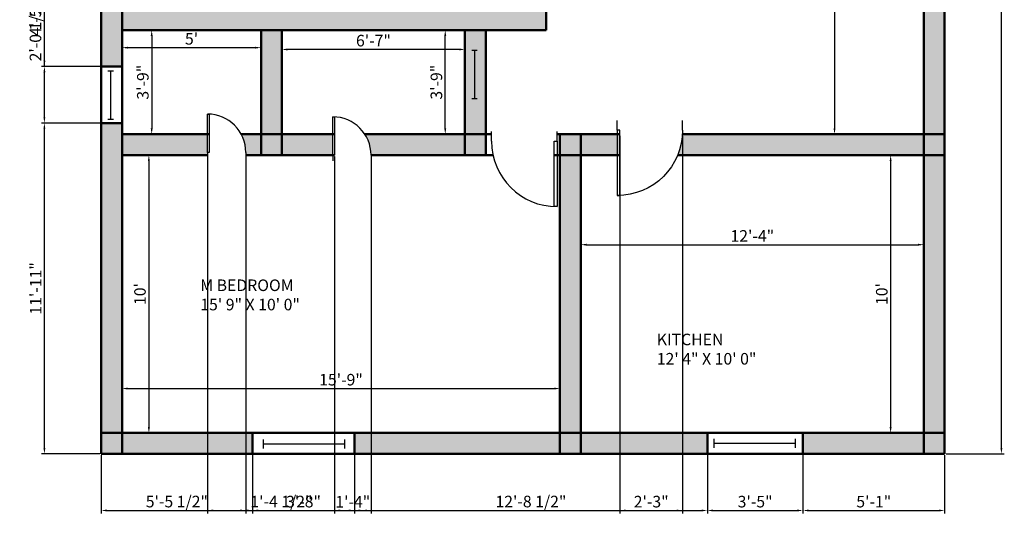
# Model space of a CAD drawing. Units: millimetres. Extents: x 2784 to 3697, y 603 to 1406.
# Tile 8 of 10: x 3272 to 3697, y 737 to 953. Entities that reach past the tile are written whole.
import ezdxf

# ---------------------------------------------------------------- set-up
doc = ezdxf.new("R2010")
doc.units = ezdxf.units.MM
for name, color, linetype, lineweight in [('A-ANNO-DIMS', 140, 'Continuous', 18), ('A-AREA-IDEN', 150, 'Continuous', 25), ('A-DOOR', 10, 'Continuous', 25), ('A-GLAZ', 30, 'Continuous', 25), ('A-WALL', 2, 'Continuous', 50), ('A-WALL-PATT', 8, 'Continuous', 13)]:
    doc.layers.add(name, color=color, linetype=linetype, lineweight=lineweight)
doc.styles.get("Standard").update_dxf_attribs({"font": 'arial.ttf'})
doc.dimstyles.new('ISO-25', dxfattribs={"dimtxt": 5, "dimasz": 2.5, "dimexe": 1.25, "dimexo": 0.625, "dimtad": 1, "dimdec": 0, "dimlunit": 3, "dimtxsty": 'Standard', "dimcen": 2.5, "dimadec": 0, "dimazin": 0, "dimtfac": 1, "dimtdec": 0, "dimtmove": 0, "dimatfit": 3, "dimfxl": 1, "dimarcsym": 0})

# ---------------------------------------------------------------- blocks, each defined once
blk = doc.blocks.new('*U2')
for p, q in [((0, 0), (0, -6)), ((40, 0), (40, -6))]:
    blk.add_line(p, q)
blk.add_lwpolyline([(0, 0), (0, 40), (1.75, 40), (1.75, 0)], close=True)
blk.add_arc((0, 0), 40, 0, 90)
blk = doc.blocks.new('*U38')
for p, q in [((0, 4), (0, 0)), ((0, 2), (36, 2)), ((36, 4), (36, 0))]:
    blk.add_line(p, q)
blk = doc.blocks.new('*D47')
at = {"layer": 'A-ANNO-DIMS', "color": 0, "lineweight": -2, "transparency": 16777216}
for p, q in [((3327.19, 894.31), (3329.06, 894.31)), ((3327.81, 891.81), (3327.81, 776.81)), ((3327.19, 774.31), (3329.06, 774.31))]:
    blk.add_line(p, q, dxfattribs=at)
at = {"layer": 'A-ANNO-DIMS', "color": 0, "transparency": 16777216}
for points in [[(3327.39, 891.81), (3328.23, 891.81), (3327.81, 894.31)], [(3327.39, 776.81), (3328.23, 776.81), (3327.81, 774.31)]]:
    blk.add_solid(points, dxfattribs=at)
at = {"layer": 'Defpoints', "color": 0, "transparency": 16777216}
for p in [(3326.56, 894.31), (3326.56, 774.31), (3327.81, 774.31)]:
    blk.add_point(p, dxfattribs=at)
at = {"layer": 'A-ANNO-DIMS', "color": 0, "transparency": 16777216, "insert": (3324.63, 834.31), "char_height": 5, "attachment_point": 5, "rotation": 90}
blk.add_mtext("10'", dxfattribs=at)
blk = doc.blocks.new('*D48')
at = {"layer": 'A-ANNO-DIMS', "color": 0, "lineweight": -2, "transparency": 16777216}
for p, q in [((3316.23, 794.11), (3316.23, 794.73)), ((3505.23, 794.11), (3505.23, 794.73)), ((3318.73, 793.48), (3502.73, 793.48))]:
    blk.add_line(p, q, dxfattribs=at)
at = {"layer": 'A-ANNO-DIMS', "color": 0, "transparency": 16777216}
for points in [[(3318.73, 793.9), (3318.73, 793.07), (3316.23, 793.48)], [(3502.73, 793.9), (3502.73, 793.07), (3505.23, 793.48)]]:
    blk.add_solid(points, dxfattribs=at)
at = {"layer": 'Defpoints', "color": 0, "transparency": 16777216}
for p in [(3316.23, 793.48), (3505.23, 793.48), (3505.23, 793.48)]:
    blk.add_point(p, dxfattribs=at)
at = {"layer": 'A-ANNO-DIMS', "color": 0, "transparency": 16777216, "insert": (3410.73, 796.66), "char_height": 5, "attachment_point": 5}
blk.add_mtext('15\'-9"', dxfattribs=at)
blk = doc.blocks.new('*D49')
at = {"layer": 'A-ANNO-DIMS', "color": 0, "lineweight": -2, "transparency": 16777216}
for p, q in [((3643.54, 894.31), (3649.17, 894.31)), ((3647.92, 891.81), (3647.92, 776.81)), ((3643.54, 774.31), (3649.17, 774.31))]:
    blk.add_line(p, q, dxfattribs=at)
at = {"layer": 'A-ANNO-DIMS', "color": 0, "transparency": 16777216}
for points in [[(3647.5, 891.81), (3648.33, 891.81), (3647.92, 894.31)], [(3647.5, 776.81), (3648.33, 776.81), (3647.92, 774.31)]]:
    blk.add_solid(points, dxfattribs=at)
at = {"layer": 'Defpoints', "color": 0, "transparency": 16777216}
for p in [(3642.91, 894.31), (3642.91, 774.31), (3647.92, 774.31)]:
    blk.add_point(p, dxfattribs=at)
at = {"layer": 'A-ANNO-DIMS', "color": 0, "transparency": 16777216, "insert": (3644.74, 834.31), "char_height": 5, "attachment_point": 5, "rotation": 90}
blk.add_mtext("10'", dxfattribs=at)
blk = doc.blocks.new('*D50')
at = {"layer": 'A-ANNO-DIMS', "color": 0, "lineweight": -2, "transparency": 16777216}
for p, q in [((3514.23, 859.71), (3514.23, 854.36)), ((3662.23, 859.71), (3662.23, 854.36)), ((3516.73, 855.61), (3659.73, 855.61))]:
    blk.add_line(p, q, dxfattribs=at)
at = {"layer": 'A-ANNO-DIMS', "color": 0, "transparency": 16777216}
for points in [[(3516.73, 856.03), (3516.73, 855.2), (3514.23, 855.61)], [(3659.73, 856.03), (3659.73, 855.2), (3662.23, 855.61)]]:
    blk.add_solid(points, dxfattribs=at)
at = {"layer": 'Defpoints', "color": 0, "transparency": 16777216}
for p in [(3514.23, 860.33), (3662.23, 860.33), (3662.23, 855.61)]:
    blk.add_point(p, dxfattribs=at)
at = {"layer": 'A-ANNO-DIMS', "color": 0, "transparency": 16777216, "insert": (3588.23, 858.75), "char_height": 5, "attachment_point": 5}
blk.add_mtext('12\'-4"', dxfattribs=at)
blk = doc.blocks.new('*D51')
at = {"layer": 'A-ANNO-DIMS', "color": 0, "lineweight": -2, "transparency": 16777216}
for p, q in [((3329.65, 948.31), (3330.28, 948.31)), ((3329.03, 945.81), (3329.03, 905.81)), ((3329.65, 903.31), (3330.28, 903.31))]:
    blk.add_line(p, q, dxfattribs=at)
at = {"layer": 'A-ANNO-DIMS', "color": 0, "transparency": 16777216}
for points in [[(3328.61, 945.81), (3329.44, 945.81), (3329.03, 948.31)], [(3328.61, 905.81), (3329.44, 905.81), (3329.03, 903.31)]]:
    blk.add_solid(points, dxfattribs=at)
at = {"layer": 'Defpoints', "color": 0, "transparency": 16777216}
for p in [(3329.03, 948.31), (3329.03, 903.31), (3329.03, 903.31)]:
    blk.add_point(p, dxfattribs=at)
at = {"layer": 'A-ANNO-DIMS', "color": 0, "transparency": 16777216, "insert": (3325.85, 925.81), "char_height": 5, "attachment_point": 5, "rotation": 90}
blk.add_mtext('3\'-9"', dxfattribs=at)
blk = doc.blocks.new('*D52')
at = {"layer": 'A-ANNO-DIMS', "color": 0, "lineweight": -2, "transparency": 16777216}
for p, q in [((3316.23, 939.95), (3316.23, 941.97)), ((3318.73, 940.72), (3373.73, 940.72)), ((3376.23, 939.95), (3376.23, 941.97))]:
    blk.add_line(p, q, dxfattribs=at)
at = {"layer": 'A-ANNO-DIMS', "color": 0, "transparency": 16777216}
for points in [[(3318.73, 941.13), (3318.73, 940.3), (3316.23, 940.72)], [(3373.73, 941.13), (3373.73, 940.3), (3376.23, 940.72)]]:
    blk.add_solid(points, dxfattribs=at)
at = {"layer": 'Defpoints', "color": 0, "transparency": 16777216}
for p in [(3316.23, 939.32), (3376.23, 940.72), (3376.23, 939.32)]:
    blk.add_point(p, dxfattribs=at)
at = {"layer": 'A-ANNO-DIMS', "color": 0, "transparency": 16777216, "insert": (3346.23, 943.89), "char_height": 5, "attachment_point": 5}
blk.add_mtext("5'", dxfattribs=at)
blk = doc.blocks.new('*D53')
at = {"layer": 'A-ANNO-DIMS', "color": 0, "lineweight": -2, "transparency": 16777216}
for p, q in [((3385.23, 941.18), (3385.23, 938.69)), ((3461.73, 939.94), (3387.73, 939.94)), ((3464.23, 941.18), (3464.23, 938.69))]:
    blk.add_line(p, q, dxfattribs=at)
at = {"layer": 'A-ANNO-DIMS', "color": 0, "transparency": 16777216}
for points in [[(3387.73, 940.36), (3387.73, 939.53), (3385.23, 939.94)], [(3461.73, 940.36), (3461.73, 939.53), (3464.23, 939.94)]]:
    blk.add_solid(points, dxfattribs=at)
at = {"layer": 'Defpoints', "color": 0, "transparency": 16777216}
for p in [(3385.23, 941.8), (3385.23, 939.94), (3464.23, 941.8)]:
    blk.add_point(p, dxfattribs=at)
at = {"layer": 'A-ANNO-DIMS', "color": 0, "transparency": 16777216, "insert": (3424.73, 943.12), "char_height": 5, "attachment_point": 5}
blk.add_mtext('6\'-7"', dxfattribs=at)
blk = doc.blocks.new('*D54')
at = {"layer": 'A-ANNO-DIMS', "color": 0, "lineweight": -2, "transparency": 16777216}
for p, q in [((3455.63, 948.31), (3454.46, 948.31)), ((3455.71, 905.81), (3455.71, 945.81)), ((3455.63, 903.31), (3454.46, 903.31))]:
    blk.add_line(p, q, dxfattribs=at)
at = {"layer": 'A-ANNO-DIMS', "color": 0, "transparency": 16777216}
for points in [[(3455.3, 945.81), (3456.13, 945.81), (3455.71, 948.31)], [(3455.3, 905.81), (3456.13, 905.81), (3455.71, 903.31)]]:
    blk.add_solid(points, dxfattribs=at)
at = {"layer": 'Defpoints', "color": 0, "transparency": 16777216}
for p in [(3455.71, 948.31), (3456.26, 948.31), (3456.26, 903.31)]:
    blk.add_point(p, dxfattribs=at)
at = {"layer": 'A-ANNO-DIMS', "color": 0, "transparency": 16777216, "insert": (3452.54, 925.81), "char_height": 5, "attachment_point": 5, "rotation": 90}
blk.add_mtext('3\'-9"', dxfattribs=at)
blk = doc.blocks.new('*D58')
at = {"layer": 'A-ANNO-DIMS', "color": 0, "lineweight": -2, "transparency": 16777216}
for p, q in [((3624.82, 1095.28), (3622.46, 1095.28)), ((3623.71, 1092.78), (3623.71, 905.81)), ((3624.82, 903.31), (3622.46, 903.31))]:
    blk.add_line(p, q, dxfattribs=at)
at = {"layer": 'A-ANNO-DIMS', "color": 0, "transparency": 16777216}
for points in [[(3623.29, 1092.78), (3624.12, 1092.78), (3623.71, 1095.28)], [(3623.29, 905.81), (3624.12, 905.81), (3623.71, 903.31)]]:
    blk.add_solid(points, dxfattribs=at)
at = {"layer": 'Defpoints', "color": 0, "transparency": 16777216}
for p in [(3625.44, 1095.28), (3623.71, 903.31), (3625.44, 903.31)]:
    blk.add_point(p, dxfattribs=at)
at = {"layer": 'A-ANNO-DIMS', "color": 0, "transparency": 16777216, "insert": (3620.53, 999.3), "char_height": 5, "attachment_point": 5, "rotation": 90}
blk.add_mtext("16'", dxfattribs=at)
blk = doc.blocks.new('*D118')
at = {"layer": 'A-ANNO-DIMS', "color": 0, "lineweight": -2, "transparency": 16777216}
for p, q in [((3307.23, 764.69), (3307.23, 739.56)), ((3372.55, 764.69), (3372.55, 739.56)), ((3309.73, 740.81), (3370.05, 740.81))]:
    blk.add_line(p, q, dxfattribs=at)
at = {"layer": 'A-ANNO-DIMS', "color": 0, "transparency": 16777216}
for points in [[(3309.73, 741.23), (3309.73, 740.39), (3307.23, 740.81)], [(3370.05, 741.23), (3370.05, 740.39), (3372.55, 740.81)]]:
    blk.add_solid(points, dxfattribs=at)
at = {"layer": 'Defpoints', "color": 0, "transparency": 16777216}
for p in [(3307.23, 765.31), (3372.55, 765.31), (3372.55, 740.81)]:
    blk.add_point(p, dxfattribs=at)
at = {"layer": 'A-ANNO-DIMS', "color": 0, "transparency": 16777216, "insert": (3339.89, 744.02), "char_height": 5, "attachment_point": 5}
blk.add_mtext('5\'-5 1/2"', dxfattribs=at)
blk = doc.blocks.new('*D119')
at = {"layer": 'A-ANNO-DIMS', "color": 0, "lineweight": -2, "transparency": 16777216}
for p, q in [((3372.55, 764.69), (3372.55, 739.56)), ((3416.56, 764.69), (3416.56, 739.56)), ((3375.05, 740.81), (3414.06, 740.81))]:
    blk.add_line(p, q, dxfattribs=at)
at = {"layer": 'A-ANNO-DIMS', "color": 0, "transparency": 16777216}
for points in [[(3375.05, 741.23), (3375.05, 740.39), (3372.55, 740.81)], [(3414.06, 741.23), (3414.06, 740.39), (3416.56, 740.81)]]:
    blk.add_solid(points, dxfattribs=at)
at = {"layer": 'Defpoints', "color": 0, "transparency": 16777216}
for p in [(3372.55, 765.31), (3416.56, 765.31), (3416.56, 740.81)]:
    blk.add_point(p, dxfattribs=at)
at = {"layer": 'A-ANNO-DIMS', "color": 0, "transparency": 16777216, "insert": (3394.55, 743.99), "char_height": 5, "attachment_point": 5}
blk.add_mtext('3\'-8"', dxfattribs=at)
blk = doc.blocks.new('*D120')
at = {"layer": 'A-ANNO-DIMS', "color": 0, "lineweight": -2, "transparency": 16777216}
for p, q in [((3416.56, 764.69), (3416.56, 739.56)), ((3568.83, 764.69), (3568.83, 739.56)), ((3419.06, 740.81), (3566.33, 740.81))]:
    blk.add_line(p, q, dxfattribs=at)
at = {"layer": 'A-ANNO-DIMS', "color": 0, "transparency": 16777216}
for points in [[(3419.06, 741.23), (3419.06, 740.39), (3416.56, 740.81)], [(3566.33, 741.23), (3566.33, 740.39), (3568.83, 740.81)]]:
    blk.add_solid(points, dxfattribs=at)
at = {"layer": 'Defpoints', "color": 0, "transparency": 16777216}
for p in [(3416.56, 765.31), (3568.83, 765.31), (3568.83, 740.81)]:
    blk.add_point(p, dxfattribs=at)
at = {"layer": 'A-ANNO-DIMS', "color": 0, "transparency": 16777216, "insert": (3492.69, 744.02), "char_height": 5, "attachment_point": 5}
blk.add_mtext('12\'-8 1/2"', dxfattribs=at)
blk = doc.blocks.new('*D121')
at = {"layer": 'A-ANNO-DIMS', "color": 0, "lineweight": -2, "transparency": 16777216}
for p, q in [((3568.83, 764.69), (3568.83, 739.56)), ((3610.06, 764.69), (3610.06, 739.56)), ((3571.33, 740.81), (3607.56, 740.81))]:
    blk.add_line(p, q, dxfattribs=at)
at = {"layer": 'A-ANNO-DIMS', "color": 0, "transparency": 16777216}
for points in [[(3571.33, 741.23), (3571.33, 740.39), (3568.83, 740.81)], [(3607.56, 741.23), (3607.56, 740.39), (3610.06, 740.81)]]:
    blk.add_solid(points, dxfattribs=at)
at = {"layer": 'Defpoints', "color": 0, "transparency": 16777216}
for p in [(3568.83, 765.31), (3610.06, 765.31), (3610.06, 740.81)]:
    blk.add_point(p, dxfattribs=at)
at = {"layer": 'A-ANNO-DIMS', "color": 0, "transparency": 16777216, "insert": (3589.44, 743.99), "char_height": 5, "attachment_point": 5}
blk.add_mtext('3\'-5"', dxfattribs=at)
blk = doc.blocks.new('*D122')
at = {"layer": 'A-ANNO-DIMS', "color": 0, "lineweight": -2, "transparency": 16777216}
for p, q in [((3610.06, 764.69), (3610.06, 739.56)), ((3671.23, 764.69), (3671.23, 739.56)), ((3612.56, 740.81), (3668.73, 740.81))]:
    blk.add_line(p, q, dxfattribs=at)
at = {"layer": 'A-ANNO-DIMS', "color": 0, "transparency": 16777216}
for points in [[(3612.56, 741.23), (3612.56, 740.39), (3610.06, 740.81)], [(3668.73, 741.23), (3668.73, 740.39), (3671.23, 740.81)]]:
    blk.add_solid(points, dxfattribs=at)
at = {"layer": 'Defpoints', "color": 0, "transparency": 16777216}
for p in [(3610.06, 765.31), (3671.23, 765.31), (3671.23, 740.81)]:
    blk.add_point(p, dxfattribs=at)
at = {"layer": 'A-ANNO-DIMS', "color": 0, "transparency": 16777216, "insert": (3640.64, 743.99), "char_height": 5, "attachment_point": 5}
blk.add_mtext('5\'-1"', dxfattribs=at)
blk = doc.blocks.new('*D123')
at = {"layer": 'A-ANNO-DIMS', "color": 0, "lineweight": -2, "transparency": 16777216}
for p, q in [((3306.6, 908.17), (3281.48, 908.17)), ((3282.73, 767.81), (3282.73, 905.67)), ((3306.6, 765.31), (3281.48, 765.31))]:
    blk.add_line(p, q, dxfattribs=at)
at = {"layer": 'A-ANNO-DIMS', "color": 0, "transparency": 16777216}
for points in [[(3282.31, 905.67), (3283.14, 905.67), (3282.73, 908.17)], [(3282.31, 767.81), (3283.14, 767.81), (3282.73, 765.31)]]:
    blk.add_solid(points, dxfattribs=at)
at = {"layer": 'Defpoints', "color": 0, "transparency": 16777216}
for p in [(3282.73, 908.17), (3307.23, 908.17), (3307.23, 765.31)]:
    blk.add_point(p, dxfattribs=at)
at = {"layer": 'A-ANNO-DIMS', "color": 0, "transparency": 16777216, "insert": (3279.59, 836.74), "char_height": 5, "attachment_point": 5, "rotation": 90}
blk.add_mtext('11\'-11"', dxfattribs=at)
blk = doc.blocks.new('*D124')
at = {"layer": 'A-ANNO-DIMS', "color": 0, "lineweight": -2, "transparency": 16777216}
for p, q in [((3282.73, 932.57), (3282.73, 961.35)), ((3306.6, 932.57), (3281.48, 932.57)), ((3282.73, 910.67), (3282.73, 930.07)), ((3306.6, 908.17), (3281.48, 908.17))]:
    blk.add_line(p, q, dxfattribs=at)
at = {"layer": 'A-ANNO-DIMS', "color": 0, "transparency": 16777216}
for points in [[(3282.31, 930.07), (3283.14, 930.07), (3282.73, 932.57)], [(3282.31, 910.67), (3283.14, 910.67), (3282.73, 908.17)]]:
    blk.add_solid(points, dxfattribs=at)
at = {"layer": 'Defpoints', "color": 0, "transparency": 16777216}
for p in [(3282.73, 932.57), (3307.23, 932.57), (3307.23, 908.17)]:
    blk.add_point(p, dxfattribs=at)
at = {"layer": 'A-ANNO-DIMS', "color": 0, "transparency": 16777216, "insert": (3279.52, 948.21), "char_height": 5, "attachment_point": 5, "rotation": 90}
blk.add_mtext('2\'-0 1/2"', dxfattribs=at)
blk = doc.blocks.new('*D125')
at = {"layer": 'A-ANNO-DIMS', "color": 0, "lineweight": -2, "transparency": 16777216}
for p, q in [((3306.6, 985.84), (3281.48, 985.84)), ((3282.73, 935.07), (3282.73, 983.34)), ((3306.6, 932.57), (3281.48, 932.57))]:
    blk.add_line(p, q, dxfattribs=at)
at = {"layer": 'A-ANNO-DIMS', "color": 0, "transparency": 16777216}
for points in [[(3282.31, 983.34), (3283.14, 983.34), (3282.73, 985.84)], [(3282.31, 935.07), (3283.14, 935.07), (3282.73, 932.57)]]:
    blk.add_solid(points, dxfattribs=at)
at = {"layer": 'Defpoints', "color": 0, "transparency": 16777216}
for p in [(3282.73, 985.84), (3307.23, 985.84), (3307.23, 932.57)]:
    blk.add_point(p, dxfattribs=at)
at = {"layer": 'A-ANNO-DIMS', "color": 0, "transparency": 16777216, "insert": (3279.52, 959.21), "char_height": 5, "attachment_point": 5, "rotation": 90}
blk.add_mtext('4\'-5 1/2"', dxfattribs=at)
blk = doc.blocks.new('*D130')
at = {"layer": 'A-ANNO-DIMS', "color": 0, "lineweight": -2, "transparency": 16777216}
for p, q in [((3671.85, 1233.28), (3696.98, 1233.28)), ((3695.73, 767.81), (3695.73, 1230.78)), ((3671.85, 765.31), (3696.98, 765.31))]:
    blk.add_line(p, q, dxfattribs=at)
at = {"layer": 'A-ANNO-DIMS', "color": 0, "transparency": 16777216}
for points in [[(3695.31, 1230.78), (3696.14, 1230.78), (3695.73, 1233.28)], [(3695.31, 767.81), (3696.14, 767.81), (3695.73, 765.31)]]:
    blk.add_solid(points, dxfattribs=at)
at = {"layer": 'Defpoints', "color": 0, "transparency": 16777216}
for p in [(3671.23, 1233.28), (3695.73, 1233.28), (3671.23, 765.31)]:
    blk.add_point(p, dxfattribs=at)
at = {"layer": 'A-ANNO-DIMS', "color": 0, "transparency": 16777216, "insert": (3692.55, 999.3), "char_height": 5, "attachment_point": 5, "rotation": 90}
blk.add_mtext('39\'-0"', dxfattribs=at)
blk = doc.blocks.new('*D136')
at = {"layer": 'A-ANNO-DIMS', "color": 0, "lineweight": -2, "transparency": 16777216}
for p, q in [((3353.12, 893.69), (3353.12, 739.56)), ((3369.65, 893.69), (3369.65, 739.56)), ((3355.62, 740.81), (3367.15, 740.81)), ((3369.65, 740.81), (3397.87, 740.81))]:
    blk.add_line(p, q, dxfattribs=at)
at = {"layer": 'A-ANNO-DIMS', "color": 0, "transparency": 16777216}
for points in [[(3355.62, 741.23), (3355.62, 740.39), (3353.12, 740.81)], [(3367.15, 741.23), (3367.15, 740.39), (3369.65, 740.81)]]:
    blk.add_solid(points, dxfattribs=at)
at = {"layer": 'Defpoints', "color": 0, "transparency": 16777216}
for p in [(3353.12, 894.31), (3369.65, 894.31), (3369.65, 740.81)]:
    blk.add_point(p, dxfattribs=at)
at = {"layer": 'A-ANNO-DIMS', "color": 0, "transparency": 16777216, "insert": (3385.01, 744.02), "char_height": 5, "attachment_point": 5}
blk.add_mtext('1\'-4 1/2"', dxfattribs=at)
blk = doc.blocks.new('*D137')
at = {"layer": 'A-ANNO-DIMS', "color": 0, "lineweight": -2, "transparency": 16777216}
for p, q in [((3407.89, 893.69), (3407.89, 739.56)), ((3423.7, 893.69), (3423.7, 739.56)), ((3410.39, 740.81), (3421.2, 740.81))]:
    blk.add_line(p, q, dxfattribs=at)
at = {"layer": 'A-ANNO-DIMS', "color": 0, "transparency": 16777216}
for points in [[(3410.39, 741.23), (3410.39, 740.39), (3407.89, 740.81)], [(3421.2, 741.23), (3421.2, 740.39), (3423.7, 740.81)]]:
    blk.add_solid(points, dxfattribs=at)
at = {"layer": 'Defpoints', "color": 0, "transparency": 16777216}
for p in [(3407.89, 894.31), (3423.7, 894.31), (3423.7, 740.81)]:
    blk.add_point(p, dxfattribs=at)
at = {"layer": 'A-ANNO-DIMS', "color": 0, "transparency": 16777216, "insert": (3415.8, 743.95), "char_height": 5, "attachment_point": 5}
blk.add_mtext('1\'-4"', dxfattribs=at)
blk = doc.blocks.new('*D138')
at = {"layer": 'A-ANNO-DIMS', "color": 0, "lineweight": -2, "transparency": 16777216}
for p, q in [((3531.12, 902.69), (3531.12, 739.56)), ((3558.05, 902.69), (3558.05, 739.56)), ((3533.62, 740.81), (3555.55, 740.81))]:
    blk.add_line(p, q, dxfattribs=at)
at = {"layer": 'A-ANNO-DIMS', "color": 0, "transparency": 16777216}
for points in [[(3533.62, 741.23), (3533.62, 740.39), (3531.12, 740.81)], [(3555.55, 741.23), (3555.55, 740.39), (3558.05, 740.81)]]:
    blk.add_solid(points, dxfattribs=at)
at = {"layer": 'Defpoints', "color": 0, "transparency": 16777216}
for p in [(3531.12, 903.31), (3558.05, 903.31), (3558.05, 740.81)]:
    blk.add_point(p, dxfattribs=at)
at = {"layer": 'A-ANNO-DIMS', "color": 0, "transparency": 16777216, "insert": (3544.59, 743.99), "char_height": 5, "attachment_point": 5}
blk.add_mtext('2\'-3"', dxfattribs=at)

msp = doc.modelspace()

# ---------------------------------------------------------------- hatches: boundary and pattern name
at = {"layer": 'A-WALL-PATT'}
h = msp.add_hatch(color=256, dxfattribs=at)
h.dxf.hatch_style = 1
h.paths.add_polyline_path([(3316.23, 1224.28), (3307.23, 1224.28), (3307.23, 1104.28), (3316.23, 1104.28)])
h.paths.add_polyline_path([(3316.23, 1233.28), (3307.23, 1233.28), (3307.23, 1224.28), (3316.23, 1224.28)])
h.paths.add_polyline_path([(3363.37, 1233.28), (3316.23, 1233.28), (3316.23, 1224.28), (3363.37, 1224.28)])
h.paths.add_polyline_path([(3460.23, 1233.28), (3405.1, 1233.28), (3405.1, 1224.28), (3460.23, 1224.28)])
h.paths.add_polyline_path([(3469.23, 1233.28), (3460.23, 1233.28), (3460.23, 1224.28), (3469.23, 1224.28)])
h.paths.add_polyline_path([(3469.23, 1224.28), (3460.23, 1224.28), (3460.23, 1104.28), (3469.23, 1104.28)])
h.paths.add_polyline_path([(3469.23, 1104.28), (3460.23, 1104.28), (3460.23, 1095.28), (3469.23, 1095.28)])
h.paths.add_polyline_path([(3460.23, 1104.28), (3444.39, 1104.28), (3444.39, 1097.52), (3444.39, 1095.28), (3460.23, 1095.28)])
h.paths.add_polyline_path([(3409.23, 1095.28), (3400.23, 1095.28), (3400.23, 1066.17, -0.119943), (3407.82, 1068.02), (3409.23, 1068.02)])
h.paths.add_polyline_path([(3409.23, 1104.28), (3400.23, 1104.28), (3400.23, 1095.28), (3409.23, 1095.28)])
h.paths.add_polyline_path([(3400.23, 1104.28), (3316.23, 1104.28), (3316.23, 1095.28), (3400.23, 1095.28)])
h.paths.add_polyline_path([(3316.23, 1104.28), (3307.23, 1104.28), (3307.23, 1095.28), (3316.23, 1095.28)])
h.paths.add_polyline_path([(3316.23, 1095.28), (3307.23, 1095.28), (3307.23, 1083.49), (3316.23, 1083.49)])
h.paths.add_polyline_path([(3416.17, 1097.52, -0.060509), (3416.99, 1104.28), (3409.23, 1104.28), (3409.23, 1095.28), (3416.17, 1095.28)])
h.paths.add_polyline_path([(3538.23, 1224.28), (3529.23, 1224.28), (3529.23, 1104.28), (3538.23, 1104.28)])
h.paths.add_polyline_path([(3538.23, 1233.28), (3529.23, 1233.28), (3529.23, 1224.28), (3538.23, 1224.28)])
h.paths.add_polyline_path([(3529.23, 1233.28), (3510.77, 1233.28), (3510.77, 1224.28), (3529.23, 1224.28)])
h.paths.add_polyline_path([(3483.89, 1233.28), (3469.23, 1233.28), (3469.23, 1224.28), (3483.89, 1224.28)])
h.paths.add_polyline_path([(3662.23, 1233.28), (3629.82, 1233.28), (3629.82, 1224.28), (3662.23, 1224.28)])
h.paths.add_polyline_path([(3671.23, 1233.28), (3662.23, 1233.28), (3662.23, 1224.28), (3671.23, 1224.28)])
h.paths.add_polyline_path([(3671.23, 1224.28), (3662.23, 1224.28), (3662.23, 1104.28), (3671.23, 1104.28)])
h.paths.add_polyline_path([(3588.37, 1233.28), (3538.23, 1233.28), (3538.23, 1224.28), (3588.37, 1224.28)])
h.paths.add_polyline_path([(3662.23, 1104.28), (3579.01, 1104.28, -0.053945), (3579.66, 1098.24), (3579.66, 1095.28), (3662.23, 1095.28)])
h.paths.add_polyline_path([(3671.23, 1104.28), (3662.23, 1104.28), (3662.23, 1095.28), (3671.23, 1095.28)])
h.paths.add_polyline_path([(3551.44, 1104.28), (3538.23, 1104.28), (3538.23, 1095.28), (3551.44, 1095.28), (3551.44, 1098.24)])
h.paths.add_polyline_path([(3538.23, 1104.28), (3529.23, 1104.28), (3529.23, 1095.28), (3538.23, 1095.28)])
h.paths.add_polyline_path([(3671.23, 1095.28), (3662.23, 1095.28), (3662.23, 903.31), (3671.23, 903.31)])
h.paths.add_polyline_path([(3316.23, 985.84), (3307.23, 985.84), (3307.23, 932.57), (3316.23, 932.57)])
h.paths.add_polyline_path([(3316.23, 1041.28), (3307.23, 1041.28), (3307.23, 1012.14), (3316.23, 1012.14)])
h.paths.add_polyline_path([(3316.23, 1050.28), (3307.23, 1050.28), (3307.23, 1041.28), (3316.23, 1041.28)])
h.paths.add_polyline_path([(3400.23, 1050.28), (3316.23, 1050.28), (3316.23, 1041.28), (3400.23, 1041.28)])
h.paths.add_polyline_path([(3316.23, 1059.19), (3307.23, 1059.19), (3307.23, 1050.28), (3316.23, 1050.28)])
h.paths.add_polyline_path([(3316.23, 908.17), (3307.23, 908.17), (3307.23, 774.31), (3316.23, 774.31)])
h.paths.add_polyline_path([(3316.23, 774.31), (3307.23, 774.31), (3307.23, 765.31), (3316.23, 765.31)])
h.paths.add_polyline_path([(3372.55, 774.31), (3316.23, 774.31), (3316.23, 765.31), (3372.55, 765.31)])
h.paths.add_polyline_path([(3505.23, 774.31), (3416.56, 774.31), (3416.56, 765.31), (3505.23, 765.31)])
h.paths.add_polyline_path([(3568.83, 774.31), (3514.23, 774.31), (3514.23, 765.31), (3568.83, 765.31)])
h.paths.add_polyline_path([(3514.23, 774.31), (3505.23, 774.31), (3505.23, 765.31), (3514.23, 765.31)])
h.paths.add_polyline_path([(3514.23, 894.31), (3505.23, 894.31), (3505.23, 774.31), (3514.23, 774.31)])
h.paths.add_polyline_path([(3514.23, 903.31), (3505.23, 903.31), (3505.23, 894.31), (3514.23, 894.31)])
h.paths.add_polyline_path([(3473.23, 948.31), (3464.23, 948.31), (3464.23, 903.31), (3473.23, 903.31)])
h.paths.add_polyline_path([(3473.23, 903.31), (3464.23, 903.31), (3464.23, 894.31), (3473.23, 894.31)])
h.paths.add_polyline_path([(3464.23, 903.31), (3421.03, 903.31, -0.144956), (3423.7, 894.31), (3464.23, 894.31)])
h.paths.add_polyline_path([(3385.23, 903.31), (3376.23, 903.31), (3376.23, 894.31), (3385.23, 894.31)])
h.paths.add_polyline_path([(3385.23, 948.31), (3376.23, 948.31), (3376.23, 903.31), (3385.23, 903.31)])
h.paths.add_polyline_path([(3407.17, 903.31), (3385.23, 903.31), (3385.23, 894.31), (3407.17, 894.31)])
h.paths.add_polyline_path([(3353.12, 903.31), (3316.23, 903.31), (3316.23, 894.31), (3353.12, 894.31), (3353.12, 895.49)])
h.paths.add_polyline_path([(3376.23, 903.31), (3367.68, 903.31, -0.123903), (3369.65, 895.49), (3369.65, 894.31), (3376.23, 894.31)])
h.paths.add_polyline_path([(3499.23, 957.31), (3499.23, 1041.28), (3490.23, 1041.28), (3490.23, 957.31), (3316.23, 957.31), (3316.23, 948.31), (3490.23, 948.31), (3499.23, 948.31)])
h.paths.add_polyline_path([(3490.23, 1050.28), (3485.56, 1050.28), (3409.23, 1050.28), (3409.23, 1041.28), (3490.23, 1041.28)])
h.paths.add_polyline_path([(3409.23, 1050.28), (3400.23, 1050.28), (3400.23, 1041.28), (3409.23, 1041.28)])
h.paths.add_polyline_path([(3499.23, 1050.28), (3490.23, 1050.28), (3490.23, 1041.28), (3499.23, 1041.28)])
h.paths.add_polyline_path([(3671.23, 894.31), (3662.23, 894.31), (3662.23, 774.31), (3671.23, 774.31)])
h.paths.add_polyline_path([(3671.23, 903.31), (3662.23, 903.31), (3662.23, 894.31), (3671.23, 894.31)])
h.paths.add_polyline_path([(3662.23, 903.31), (3558.05, 903.31, -0.082354), (3555.98, 894.31), (3662.23, 894.31)])
h.paths.add_polyline_path([(3529.88, 903.31), (3514.23, 903.31), (3514.23, 894.31), (3529.88, 894.31)])
h.paths.add_polyline_path([(3531.12, 903.31), (3529.88, 903.31), (3529.88, 894.31), (3531.12, 894.31)])
h.paths.add_polyline_path([(3662.23, 774.31), (3610.06, 774.31), (3610.06, 765.31), (3662.23, 765.31)])
h.paths.add_polyline_path([(3671.23, 774.31), (3662.23, 774.31), (3662.23, 765.31), (3671.23, 765.31)])
h.paths.add_polyline_path([(3544.99, 801.01), (3590.84, 801.01), (3590.84, 819.67), (3544.99, 819.67)], flags=9)
h.paths.add_polyline_path([(3347.99, 824.43), (3394.58, 824.43), (3394.58, 843.09), (3347.99, 843.09)], flags=9)
h.paths.add_polyline_path([(3546.35, 988.53), (3592.21, 988.53), (3592.21, 1007.19), (3546.35, 1007.19)], flags=9)
h.paths.add_polyline_path([(3329.63, 1060.44), (3367.72, 1060.44), (3367.72, 1079.1), (3329.63, 1079.1)], flags=9)
h.paths.add_polyline_path([(3353.92, 1169.75), (3400.92, 1169.75), (3400.92, 1188.4), (3353.92, 1188.4)], flags=9)

# ---------------------------------------------------------------- linework, layer by layer
at = {"layer": 'A-WALL'}
for p, q in [((3307.23, 1233.28), (3307.23, 765.31)), ((3316.23, 1233.28), (3316.23, 765.31)), ((3662.23, 1233.28), (3662.23, 765.31)), ((3671.23, 1233.28), (3671.23, 765.31)), ((3499.23, 948.31), (3499.23, 957.31)), ((3316.23, 948.31), (3490.23, 948.31)), ((3376.23, 948.31), (3376.23, 894.31)), ((3385.23, 948.31), (3385.23, 894.31)), ((3464.23, 948.31), (3464.23, 894.31)), ((3473.23, 948.31), (3473.23, 894.31)), ((3490.23, 948.31), (3499.23, 948.31)), ((3316.23, 932.57), (3307.23, 932.57)), ((3316.23, 908.17), (3307.23, 908.17)), ((3316.23, 903.31), (3353.84, 903.31)), ((3367.68, 903.31), (3407.89, 903.31)), ((3421.03, 903.31), (3475.73, 903.31)), ((3503.95, 903.31), (3531.12, 903.31)), ((3505.23, 903.31), (3505.23, 765.31)), ((3514.23, 903.31), (3514.23, 765.31)), ((3558.05, 903.31), (3671.23, 903.31)), ((3316.23, 894.31), (3353.12, 894.31)), ((3369.65, 894.31), (3407.89, 894.31)), ((3423.7, 894.31), (3476.36, 894.31)), ((3502.72, 894.31), (3531.12, 894.31)), ((3555.98, 894.31), (3671.23, 894.31)), ((3307.23, 774.31), (3671.23, 774.31)), ((3372.55, 774.31), (3372.55, 765.31)), ((3416.56, 774.31), (3416.56, 765.31)), ((3568.83, 774.31), (3568.83, 765.31)), ((3610.06, 774.31), (3610.06, 765.31)), ((3307.23, 765.31), (3671.23, 765.31))]:
    msp.add_line(p, q, dxfattribs=at)

# ---------------------------------------------------------------- block references
at = {"layer": 'A-DOOR', "xscale": 0.413209421180039, "yscale": 0.413209421180039, "zscale": 0.413209421180039}
for p in [(3353.12, 895.49), (3407.17, 894.31)]:
    msp.add_blockref('*U2', p, dxfattribs=at)
at = {"layer": 'A-DOOR', "yscale": 0.7055841571326333, "zscale": 0.7055841571326333, "rotation": 180}
for p, xscale in [((3529.88, 905.05), -0.7055841571326333), ((3503.95, 900.27), 0.7055841571326333)]:
    msp.add_blockref('*U2', p, dxfattribs=dict(at, xscale=xscale))
at = {"layer": 'A-GLAZ', "xscale": 0.5811470115210491, "yscale": 0.5811470115210491, "zscale": 0.5811470115210491, "rotation": 269.9999999999999}
for p in [(3467.2, 939.55), (3310.15, 930.58)]:
    msp.add_blockref('*U38', p, dxfattribs=at)
at = {"layer": 'A-GLAZ', "xscale": 0.9748873049904094, "yscale": 0.9748873049904094, "zscale": 0.9748873049904094}
for p in [(3377.12, 767.64), (3571.6, 767.93)]:
    msp.add_blockref('*U38', p, dxfattribs=at)

# ---------------------------------------------------------------- texts
at = {"layer": 'A-AREA-IDEN', "char_height": 5, "attachment_point": 1}
for s, width, insert in [('M BEDROOM \\P15\' 9" X 10\' 0"', 131.4901, (3350, 840.6)), ('KITCHEN \\P12\' 4" X 10\' 0"', 63.7234, (3547, 817.18))]:
    msp.add_mtext_dynamic_manual_height_columns(s, width=width, gutter_width=12.5, heights=[0], dxfattribs=dict(at, insert=insert))

# ---------------------------------------------------------------- dimensions: what is measured, and where the dimension line sits
at = {"layer": 'A-ANNO-DIMS'}
for base, p1, p2, override, picture, middle in [((3695.73, 1233.28), (3671.23, 765.31), (3671.23, 1233.28), {"dimdec": 1, "dimlfac": 1, "dimrnd": 0, "dimzin": 1, "dimdsep": 46, "dimlunit": 4, "dimfrac": 2}, '*D130', (3692.55, 999.3)), ((3623.71, 903.31), (3625.44, 1095.28), (3625.44, 903.31), {"dimclrd": 0, "dimclre": 0, "dimclrt": 0}, '*D58', (3620.53, 999.3)), ((3282.73, 985.84), (3307.23, 932.57), (3307.23, 985.84), {"dimdec": 1, "dimlfac": 1, "dimrnd": 0, "dimzin": 1, "dimdsep": 46, "dimlunit": 4, "dimfrac": 2}, '*D125', (3279.52, 959.21)), ((3282.73, 932.57), (3307.23, 908.17), (3307.23, 932.57), {"dimdec": 1, "dimlfac": 1, "dimrnd": 0, "dimzin": 1, "dimdsep": 46, "dimlunit": 4, "dimfrac": 2}, '*D124', (3279.52, 948.21)), ((3329.03, 903.31), (3329.03, 948.31), (3329.03, 903.31), {"dimclrd": 0, "dimclre": 0, "dimclrt": 0}, '*D51', (3325.85, 925.81)), ((3455.71, 948.31), (3456.26, 903.31), (3456.26, 948.31), {"dimclrd": 0, "dimclre": 0, "dimclrt": 0}, '*D54', (3452.54, 925.81)), ((3282.73, 908.17), (3307.23, 765.31), (3307.23, 908.17), {"dimdec": 1, "dimlfac": 1, "dimrnd": 0, "dimzin": 1, "dimdsep": 46, "dimlunit": 4, "dimfrac": 2}, '*D123', (3279.59, 836.74)), ((3327.81, 774.31), (3326.56, 894.31), (3326.56, 774.31), {"dimclrd": 0, "dimclre": 0, "dimclrt": 0}, '*D47', (3324.63, 834.31)), ((3647.92, 774.31), (3642.91, 894.31), (3642.91, 774.31), {"dimclrd": 0, "dimclre": 0, "dimclrt": 0}, '*D49', (3644.74, 834.31))]:
    dim = msp.add_linear_dim(base=base, p1=p1, p2=p2, angle=90, dimstyle='ISO-25', override=override, dxfattribs=at)
    dim.commit()
    dim.dimension.update_dxf_attribs({"geometry": picture, "text_midpoint": middle})
for base, p1, p2, override, picture, middle in [((3376.23, 940.72), (3316.23, 939.32), (3376.23, 939.32), {"dimclrd": 0, "dimclre": 0, "dimclrt": 0}, '*D52', (3346.23, 943.89)), ((3385.23, 939.94), (3464.23, 941.8), (3385.23, 941.8), {"dimclrd": 0, "dimclre": 0, "dimclrt": 0}, '*D53', (3424.73, 943.12)), ((3558.05, 740.81), (3531.12, 903.31), (3558.05, 903.31), {"dimdec": 1, "dimlfac": 1, "dimrnd": 0, "dimzin": 1, "dimdsep": 46, "dimlunit": 4, "dimfrac": 2}, '*D138', (3544.59, 743.99)), ((3369.65, 740.81), (3353.12, 894.31), (3369.65, 894.31), {"dimdec": 1, "dimlfac": 1, "dimrnd": 0, "dimzin": 1, "dimdsep": 46, "dimlunit": 4, "dimfrac": 2}, '*D136', (3385.01, 744.02)), ((3423.7, 740.81), (3407.89, 894.31), (3423.7, 894.31), {"dimdec": 1, "dimlfac": 1, "dimrnd": 0, "dimzin": 1, "dimdsep": 46, "dimlunit": 4, "dimfrac": 2}, '*D137', (3415.8, 743.95)), ((3662.23, 855.61), (3514.23, 860.33), (3662.23, 860.33), {"dimclrd": 0, "dimclre": 0, "dimclrt": 0}, '*D50', (3588.23, 858.75)), ((3505.23, 793.48), (3316.23, 793.48), (3505.23, 793.48), {"dimclrd": 0, "dimclre": 0, "dimclrt": 0}, '*D48', (3410.73, 796.66)), ((3372.55, 740.81), (3307.23, 765.31), (3372.55, 765.31), {"dimdec": 1, "dimlfac": 1, "dimrnd": 0, "dimzin": 1, "dimdsep": 46, "dimlunit": 4, "dimfrac": 2}, '*D118', (3339.89, 744.02)), ((3416.56, 740.81), (3372.55, 765.31), (3416.56, 765.31), {"dimdec": 1, "dimlfac": 1, "dimrnd": 0, "dimzin": 1, "dimdsep": 46, "dimlunit": 4, "dimfrac": 2}, '*D119', (3394.55, 743.99)), ((3568.83, 740.81), (3416.56, 765.31), (3568.83, 765.31), {"dimdec": 1, "dimlfac": 1, "dimrnd": 0, "dimzin": 1, "dimdsep": 46, "dimlunit": 4, "dimfrac": 2}, '*D120', (3492.69, 744.02)), ((3610.06, 740.81), (3568.83, 765.31), (3610.06, 765.31), {"dimdec": 1, "dimlfac": 1, "dimrnd": 0, "dimzin": 1, "dimdsep": 46, "dimlunit": 4, "dimfrac": 2}, '*D121', (3589.44, 743.99)), ((3671.23, 740.81), (3610.06, 765.31), (3671.23, 765.31), {"dimdec": 1, "dimlfac": 1, "dimrnd": 0, "dimzin": 1, "dimdsep": 46, "dimlunit": 4, "dimfrac": 2}, '*D122', (3640.64, 743.99))]:
    dim = msp.add_linear_dim(base=base, p1=p1, p2=p2, dimstyle='ISO-25', override=override, dxfattribs=at)
    dim.commit()
    dim.dimension.update_dxf_attribs({"geometry": picture, "text_midpoint": middle})

doc.saveas('drawing.dxf')
